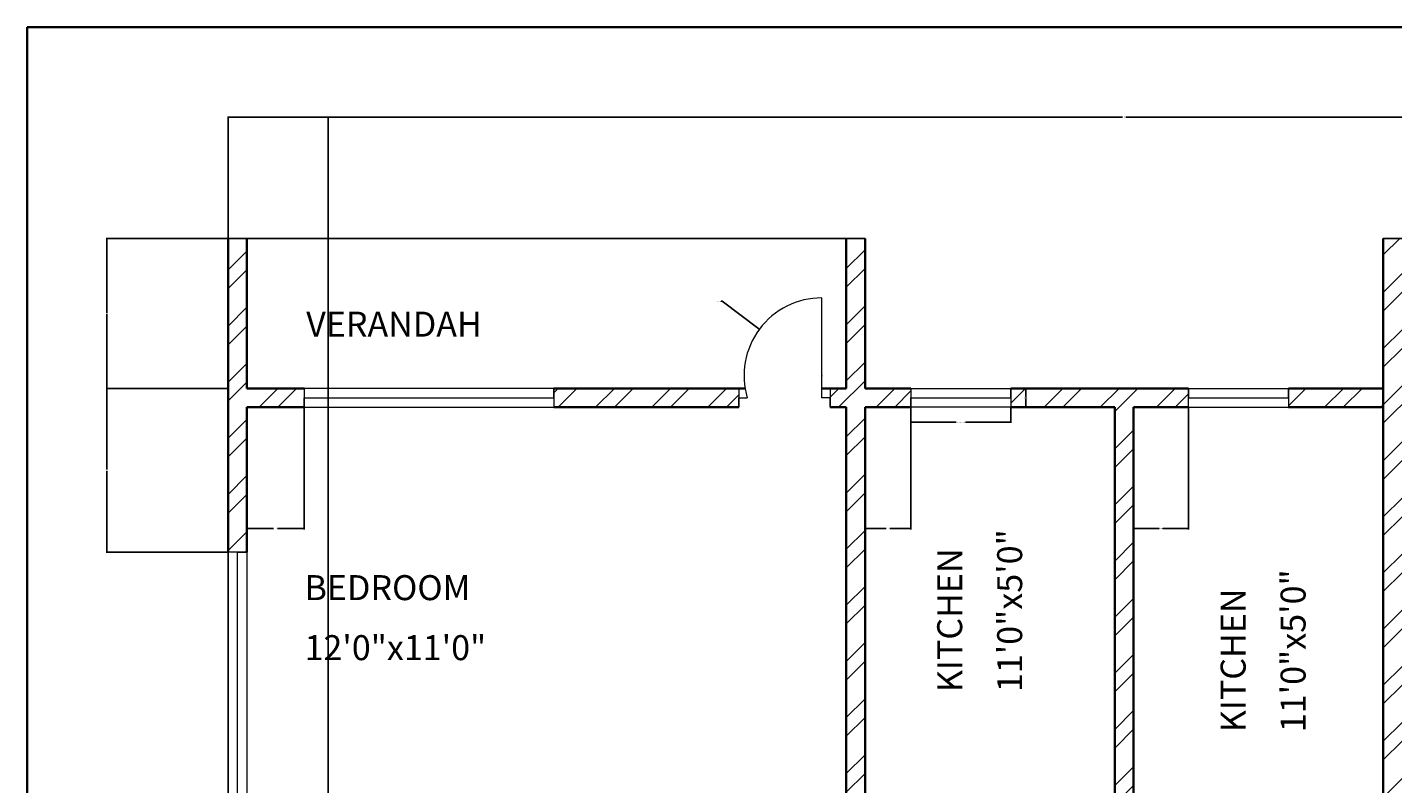
# Model space of a CAD drawing. Units: inches. Extents: x 2271 to 2815, y 1169 to 1838.
# Tile 3 of 4: x 2271 to 2599, y 1657 to 1838. Entities that reach past the tile are written whole.
import ezdxf

# ---------------------------------------------------------------- set-up
doc = ezdxf.new("R2010")
doc.units = ezdxf.units.IN
for name, color, linetype, lineweight in [('A-ANNO-DIMS', 2, 'Continuous', 18), ('A-ANNO-TTLB', 7, 'Continuous', 35), ('A-AREA-IDEN', 7, 'Continuous', 18), ('A-DOOR', 11, 'Continuous', 18), ('A-FLOR-EDGE', 7, 'Continuous', 25), ('A-GLAZ', 181, 'Continuous', 18), ('A-WALL', 7, 'Continuous', 35)]:
    doc.layers.add(name, color=color, linetype=linetype, lineweight=lineweight)
doc.layers.add('A-WALL-PATT', color=9, linetype='Continuous', lineweight=13, true_color=0xafd9aa)
doc.styles.get("Standard").update_dxf_attribs({"font": 'arial.ttf'})
doc.dimstyles.get("Standard").update_dxf_attribs({"dimtxt": 0.18, "dimasz": 0.18, "dimexe": 0.18, "dimexo": 0.0625, "dimgap": 0.09, "dimtad": 0, "dimtih": 1, "dimtoh": 1, "dimdec": 4, "dimzin": 0, "dimdsep": 46, "dimtxsty": 'Standard', "dimcen": 0.09, "dimadec": 0, "dimazin": 0, "dimtfac": 1, "dimtdec": 4, "dimtofl": 0, "dimtmove": 0, "dimatfit": 3, "dimfxl": 1, "dimtolj": 1, "dimtzin": 0, "dimarcsym": 0})

# ---------------------------------------------------------------- blocks, each defined once
blk = doc.blocks.new('WIN-60IN')
for p, q in [((0, 4.5), (0, 0)), ((60, 4.5), (0, 4.5)), ((60, 2.25), (60, 4.5)), ((60, 4.5), (60, 0)), ((0, 0), (0, 2.25)), ((0, 2.25), (60, 2.25)), ((0, 0), (60, 0))]:
    blk.add_line(p, q)
blk = doc.blocks.new('WIN-24IN')
for p, q in [((0, 4.5), (0, 0)), ((0, 4.5), (24, 4.5)), ((24, 2.25), (24, 4.5)), ((24, 4.5), (24, 0)), ((0, 0), (0, 2.25)), ((0, 2.25), (24, 2.25)), ((24, 0), (0, 0))]:
    blk.add_line(p, q)
blk = doc.blocks.new('*D5')
at = {"layer": 'A-ANNO-DIMS', "color": 0, "lineweight": -2, "transparency": 16777216}
for p, q in [((2482.83, 1746.97), (2482.83, 1743.25)), ((2506.83, 1746.97), (2506.83, 1743.25)), ((2483.01, 1743.43), (2493.71, 1743.43)), ((2506.65, 1743.43), (2495.95, 1743.43))]:
    blk.add_line(p, q, dxfattribs=at)
at = {"layer": 'A-ANNO-DIMS', "color": 0, "transparency": 16777216}
for points in [[(2483.01, 1743.46), (2483.01, 1743.4), (2482.83, 1743.43)], [(2506.65, 1743.46), (2506.65, 1743.4), (2506.83, 1743.43)]]:
    blk.add_solid(points, dxfattribs=at)
at = {"layer": 'Defpoints', "color": 0, "transparency": 16777216}
for p in [(2482.83, 1747.03), (2506.83, 1747.03), (2506.83, 1743.43)]:
    blk.add_point(p, dxfattribs=at)
at = {"layer": 'A-ANNO-DIMS', "color": 0, "transparency": 16777216, "insert": (2494.83, 1743.43), "char_height": 0.18, "attachment_point": 5}
blk.add_mtext('\\A1;WINDOW 24 TYP.', dxfattribs=at)
blk = doc.blocks.new('*D6')
at = {"layer": 'A-ANNO-DIMS', "color": 0, "lineweight": -2, "transparency": 16777216}
for p, q in [((2506.89, 1751.53), (2510.61, 1751.53)), ((2510.43, 1751.35), (2510.43, 1749.46)), ((2510.43, 1747.21), (2510.43, 1749.1)), ((2506.89, 1747.03), (2510.61, 1747.03))]:
    blk.add_line(p, q, dxfattribs=at)
at = {"layer": 'A-ANNO-DIMS', "color": 0, "transparency": 16777216}
for points in [[(2510.4, 1751.35), (2510.46, 1751.35), (2510.43, 1751.53)], [(2510.4, 1747.21), (2510.46, 1747.21), (2510.43, 1747.03)]]:
    blk.add_solid(points, dxfattribs=at)
at = {"layer": 'Defpoints', "color": 0, "transparency": 16777216}
for p in [(2506.83, 1751.53), (2510.43, 1751.53), (2506.83, 1747.03)]:
    blk.add_point(p, dxfattribs=at)
at = {"layer": 'A-ANNO-DIMS', "color": 0, "transparency": 16777216, "insert": (2510.43, 1749.28), "char_height": 0.18, "attachment_point": 5}
blk.add_mtext('\\A1;5 TYP.', dxfattribs=at)
blk = doc.blocks.new('*D7')
at = {"layer": 'A-ANNO-DIMS', "color": 0, "lineweight": -2, "transparency": 16777216}
for p, q in [((2318.8, 1787.59), (2318.8, 1816.86)), ((2318.98, 1816.68), (2533.65, 1816.68)), ((2749.12, 1816.68), (2534.45, 1816.68)), ((2749.3, 1787.59), (2749.3, 1816.86))]:
    blk.add_line(p, q, dxfattribs=at)
at = {"layer": 'A-ANNO-DIMS', "color": 0, "transparency": 16777216}
for points in [[(2318.98, 1816.71), (2318.98, 1816.65), (2318.8, 1816.68)], [(2749.12, 1816.71), (2749.12, 1816.65), (2749.3, 1816.68)]]:
    blk.add_solid(points, dxfattribs=at)
at = {"layer": 'Defpoints', "color": 0, "transparency": 16777216}
for p in [(2749.3, 1816.68), (2318.8, 1787.53), (2749.3, 1787.53)]:
    blk.add_point(p, dxfattribs=at)
at = {"layer": 'A-ANNO-DIMS', "color": 0, "transparency": 16777216, "insert": (2534.05, 1816.68), "char_height": 0.18, "attachment_point": 5}
blk.add_mtext('\\A1;430.5', dxfattribs=at)
blk = doc.blocks.new('*D21')
at = {"layer": 'A-ANNO-DIMS', "color": 0, "lineweight": -2, "transparency": 16777216}
for p, q in [((2318.74, 1751.53), (2289.47, 1751.53)), ((2289.65, 1751.35), (2289.65, 1732.06)), ((2289.65, 1712.4), (2289.65, 1731.69)), ((2318.74, 1712.22), (2289.47, 1712.22))]:
    blk.add_line(p, q, dxfattribs=at)
at = {"layer": 'A-ANNO-DIMS', "color": 0, "transparency": 16777216}
for points in [[(2289.62, 1751.35), (2289.68, 1751.35), (2289.65, 1751.53)], [(2289.62, 1712.4), (2289.68, 1712.4), (2289.65, 1712.22)]]:
    blk.add_solid(points, dxfattribs=at)
at = {"layer": 'Defpoints', "color": 0, "transparency": 16777216}
for p in [(2289.65, 1751.53), (2318.8, 1751.53), (2318.8, 1712.22)]:
    blk.add_point(p, dxfattribs=at)
at = {"layer": 'A-ANNO-DIMS', "color": 0, "transparency": 16777216, "insert": (2289.65, 1731.87), "char_height": 0.18, "attachment_point": 5}
blk.add_mtext('\\A1;39.31', dxfattribs=at)
blk = doc.blocks.new('*D22')
at = {"layer": 'A-ANNO-DIMS', "color": 0, "lineweight": -2, "transparency": 16777216}
for p, q in [((2318.74, 1787.53), (2289.47, 1787.53)), ((2289.65, 1787.35), (2289.65, 1769.71)), ((2289.65, 1751.71), (2289.65, 1769.35)), ((2318.74, 1751.53), (2289.47, 1751.53))]:
    blk.add_line(p, q, dxfattribs=at)
at = {"layer": 'A-ANNO-DIMS', "color": 0, "transparency": 16777216}
for points in [[(2289.62, 1787.35), (2289.68, 1787.35), (2289.65, 1787.53)], [(2289.62, 1751.71), (2289.68, 1751.71), (2289.65, 1751.53)]]:
    blk.add_solid(points, dxfattribs=at)
at = {"layer": 'Defpoints', "color": 0, "transparency": 16777216}
for p in [(2289.65, 1787.53), (2318.8, 1787.53), (2318.8, 1751.53)]:
    blk.add_point(p, dxfattribs=at)
at = {"layer": 'A-ANNO-DIMS', "color": 0, "transparency": 16777216, "insert": (2289.65, 1769.53), "char_height": 0.18, "attachment_point": 5}
blk.add_mtext('\\A1;36', dxfattribs=at)
blk = doc.blocks.new('*D23')
at = {"layer": 'A-ANNO-DIMS', "color": 0, "lineweight": -2, "transparency": 16777216}
for p, q in [((2318.8, 1433.59), (2318.8, 1816.86)), ((2318.98, 1816.68), (2330.58, 1816.68)), ((2342.62, 1816.68), (2331.02, 1816.68)), ((2342.8, 1433.59), (2342.8, 1816.86))]:
    blk.add_line(p, q, dxfattribs=at)
at = {"layer": 'A-ANNO-DIMS', "color": 0, "transparency": 16777216}
for points in [[(2318.98, 1816.71), (2318.98, 1816.65), (2318.8, 1816.68)], [(2342.62, 1816.71), (2342.62, 1816.65), (2342.8, 1816.68)]]:
    blk.add_solid(points, dxfattribs=at)
at = {"layer": 'Defpoints', "color": 0, "transparency": 16777216}
for p in [(2342.8, 1816.68), (2318.8, 1433.53), (2342.8, 1433.53)]:
    blk.add_point(p, dxfattribs=at)
at = {"layer": 'A-ANNO-DIMS', "color": 0, "transparency": 16777216, "insert": (2330.8, 1816.68), "char_height": 0.18, "attachment_point": 5}
blk.add_mtext('\\A1;24', dxfattribs=at)
blk = doc.blocks.new('*D26')
at = {"layer": 'A-ANNO-DIMS', "color": 0, "lineweight": -2, "transparency": 16777216}
for p, q in [((2323.3, 1746.97), (2323.3, 1717.7)), ((2337.06, 1746.97), (2337.06, 1717.7)), ((2323.48, 1717.88), (2329.72, 1717.88)), ((2336.88, 1717.88), (2330.63, 1717.88))]:
    blk.add_line(p, q, dxfattribs=at)
at = {"layer": 'A-ANNO-DIMS', "color": 0, "transparency": 16777216}
for points in [[(2323.48, 1717.91), (2323.48, 1717.85), (2323.3, 1717.88)], [(2336.88, 1717.91), (2336.88, 1717.85), (2337.06, 1717.88)]]:
    blk.add_solid(points, dxfattribs=at)
at = {"layer": 'Defpoints', "color": 0, "transparency": 16777216}
for p in [(2323.3, 1747.03), (2337.06, 1747.03), (2323.3, 1717.88)]:
    blk.add_point(p, dxfattribs=at)
at = {"layer": 'A-ANNO-DIMS', "color": 0, "transparency": 16777216, "insert": (2330.18, 1717.88), "char_height": 0.18, "attachment_point": 5}
blk.add_mtext('\\A1;13.757', dxfattribs=at)
blk = doc.blocks.new('*D27')
at = {"layer": 'A-ANNO-DIMS', "color": 0, "lineweight": -2, "transparency": 16777216}
for p, q in [((2471.8, 1746.97), (2471.8, 1717.7)), ((2482.83, 1746.97), (2482.83, 1717.7)), ((2471.98, 1717.88), (2476.86, 1717.88)), ((2482.65, 1717.88), (2477.77, 1717.88))]:
    blk.add_line(p, q, dxfattribs=at)
at = {"layer": 'A-ANNO-DIMS', "color": 0, "transparency": 16777216}
for points in [[(2471.98, 1717.91), (2471.98, 1717.85), (2471.8, 1717.88)], [(2482.65, 1717.91), (2482.65, 1717.85), (2482.83, 1717.88)]]:
    blk.add_solid(points, dxfattribs=at)
at = {"layer": 'Defpoints', "color": 0, "transparency": 16777216}
for p in [(2471.8, 1747.03), (2482.83, 1747.03), (2471.8, 1717.88)]:
    blk.add_point(p, dxfattribs=at)
at = {"layer": 'A-ANNO-DIMS', "color": 0, "transparency": 16777216, "insert": (2477.31, 1717.88), "char_height": 0.18, "attachment_point": 5}
blk.add_mtext('\\A1;11.027', dxfattribs=at)
blk = doc.blocks.new('*D28')
at = {"layer": 'A-ANNO-DIMS', "color": 0, "lineweight": -2, "transparency": 16777216}
for p, q in [((2536.3, 1746.97), (2536.3, 1717.7)), ((2549.52, 1746.97), (2549.52, 1717.7)), ((2536.48, 1717.88), (2542.45, 1717.88)), ((2549.34, 1717.88), (2543.36, 1717.88))]:
    blk.add_line(p, q, dxfattribs=at)
at = {"layer": 'A-ANNO-DIMS', "color": 0, "transparency": 16777216}
for points in [[(2536.48, 1717.91), (2536.48, 1717.85), (2536.3, 1717.88)], [(2549.34, 1717.91), (2549.34, 1717.85), (2549.52, 1717.88)]]:
    blk.add_solid(points, dxfattribs=at)
at = {"layer": 'Defpoints', "color": 0, "transparency": 16777216}
for p in [(2536.3, 1747.03), (2549.52, 1747.03), (2536.3, 1717.88)]:
    blk.add_point(p, dxfattribs=at)
at = {"layer": 'A-ANNO-DIMS', "color": 0, "transparency": 16777216, "insert": (2542.91, 1717.88), "char_height": 0.18, "attachment_point": 5}
blk.add_mtext('\\A1;13.218', dxfattribs=at)
blk = doc.blocks.new('*D46')
at = {"layer": 'A-ANNO-DIMS', "color": 0, "lineweight": -2, "transparency": 16777216}
for p, q in [((2437.27, 1772.48), (2437.45, 1772.48)), ((2437.45, 1772.48), (2446.29, 1765.88)), ((2461.32, 1754.59), (2461.5, 1754.59)), ((2461.41, 1754.5), (2461.41, 1754.68))]:
    blk.add_line(p, q, dxfattribs=at)
at = {"layer": 'A-ANNO-DIMS', "color": 0, "transparency": 16777216}
blk.add_solid([(2446.31, 1765.91), (2446.27, 1765.86), (2446.44, 1765.77)], dxfattribs=at)
at = {"layer": 'Defpoints', "color": 0, "transparency": 16777216}
for p in [(2446.44, 1765.77), (2461.41, 1754.59)]:
    blk.add_point(p, dxfattribs=at)
at = {"layer": 'A-ANNO-DIMS', "color": 0, "transparency": 16777216, "insert": (2436.79, 1772.48), "char_height": 0.18, "attachment_point": 5}
blk.add_mtext('\\A1;R18.69', dxfattribs=at)

msp = doc.modelspace()

# ---------------------------------------------------------------- hatches: boundary and pattern name
at = {"layer": 'A-WALL-PATT'}
h = msp.add_hatch(dxfattribs=at)
h.set_pattern_fill('ANSI32', color=256)
h.paths.add_polyline_path([(2441.4917, 1751.5314), (2397.0578, 1751.5314), (2397.0578, 1747.0314), (2441.4917, 1747.0314), (2441.4917, 1749.2814)])
h.paths.add_polyline_path([(2471.8006, 1787.5314), (2467.3006, 1787.5314), (2467.3006, 1783.0314), (2467.3006, 1751.5314), (2463.4131, 1751.5314), (2463.4131, 1747.0314), (2467.3006, 1747.0314), (2467.3006, 1615.0314), (2465.0606, 1615.0314), (2465.0606, 1610.5314), (2474.7192, 1610.5314), (2474.7192, 1612.7814), (2474.7192, 1615.0314), (2471.8006, 1615.0314), (2471.8006, 1747.0314), (2482.8275, 1747.0314), (2482.8275, 1749.2814), (2482.8275, 1751.5314), (2471.8006, 1751.5314)])
h.paths.add_polyline_path([(2549.5185, 1751.5314), (2506.8275, 1751.5314), (2506.8275, 1747.0314), (2531.8006, 1747.0314), (2531.8006, 1615.0314), (2496.0724, 1615.0314), (2496.0724, 1610.5314), (2531.8006, 1610.5314), (2531.8006, 1458.2548), (2528.7405, 1458.2548), (2528.7405, 1453.7548), (2539.7806, 1453.7548), (2539.7806, 1456.0048), (2539.7806, 1458.2548), (2536.3006, 1458.2548), (2536.3006, 1610.5314), (2573.267, 1610.5314), (2573.267, 1612.5736), (2573.267, 1612.7912), (2573.267, 1615.0314), (2536.3006, 1615.0314), (2536.3006, 1747.0314), (2549.5185, 1747.0314)])
h.paths.add_polyline_path([(2600.8006, 1787.5314), (2596.3006, 1787.5314), (2596.3006, 1747.0314), (2596.3006, 1615.0314), (2593.1473, 1615.0314), (2593.1473, 1610.5314), (2603.416, 1610.5314), (2603.416, 1612.7814), (2603.416, 1615.0314), (2600.8006, 1615.0314), (2600.8006, 1747.0314), (2603.7892, 1747.0314), (2603.7892, 1749.2814), (2603.7892, 1751.5314), (2600.8006, 1751.5314)])
h.paths.add_polyline_path([(2596.3006, 1751.5314), (2573.5185, 1751.5314), (2573.5185, 1747.0314), (2596.3006, 1747.0314)])
h.paths.add_polyline_path([(2648.9302, 1749.2814), (2648.9302, 1751.5314), (2624.6394, 1751.5314), (2624.6394, 1747.0314), (2648.9302, 1747.0314)])
h.paths.add_polyline_path([(2749.3006, 1751.5314), (2749.3006, 1787.5314), (2744.8006, 1787.5314), (2744.8006, 1751.5314), (2708.9302, 1751.5314), (2708.9302, 1747.0314), (2744.8006, 1747.0314), (2744.8006, 1715.8571), (2749.3006, 1715.8571)])
h.paths.add_polyline_path([(2337.0578, 1749.2814), (2337.0578, 1751.5314), (2323.3006, 1751.5314), (2323.3006, 1787.5314), (2318.8006, 1787.5314), (2318.8006, 1751.5314), (2318.8006, 1712.2179), (2323.3006, 1712.2179), (2323.3006, 1747.0314), (2337.0578, 1747.0314)])
h.paths.add_polyline_path([(2402.757, 1615.0314), (2323.3006, 1615.0314), (2323.3006, 1652.2179), (2318.8006, 1652.2179), (2318.8006, 1610.5314), (2323.3006, 1610.5314), (2342.8006, 1610.5314), (2342.8006, 1602.42), (2347.3006, 1602.42), (2347.3006, 1610.5314), (2402.757, 1610.5314)])
h.paths.add_polyline_path([(2430.8006, 1568.5314), (2430.8006, 1610.5314), (2434.8435, 1610.5314), (2434.8435, 1612.7814), (2434.8435, 1615.0314), (2422.3947, 1615.0314), (2422.3947, 1612.7814), (2422.3947, 1610.5314), (2426.3006, 1610.5314), (2426.3006, 1568.5314), (2347.3006, 1568.5314), (2347.3006, 1578.42), (2342.8006, 1578.42), (2342.8006, 1568.5314), (2318.8006, 1568.5314), (2318.8006, 1546.0693), (2322.7121, 1546.0693), (2323.3006, 1546.0693), (2323.3006, 1564.0314), (2342.8006, 1564.0314), (2347.3006, 1564.0314), (2430.8006, 1564.0314)])
h.paths.add_polyline_path([(2430.8006, 1480.0314), (2323.3006, 1480.0314), (2323.3006, 1498.0693), (2321.0506, 1498.0693), (2318.8006, 1498.0693), (2318.8006, 1475.5314), (2342.8006, 1475.5314), (2342.8006, 1466.8218), (2347.3006, 1466.8218), (2347.3006, 1475.5314), (2426.3006, 1475.5314), (2426.3006, 1458.0149), (2430.8006, 1458.0149), (2430.8006, 1475.5314)])
h.paths.add_polyline_path([(2435.9471, 1433.5314), (2430.8006, 1433.5314), (2430.8006, 1437.7896), (2426.3006, 1437.7896), (2426.3006, 1433.5314), (2347.3006, 1433.5314), (2347.3006, 1442.8218), (2342.8006, 1442.8218), (2342.8006, 1433.5314), (2318.8006, 1433.5314), (2318.8006, 1402.3145), (2323.3006, 1402.3145), (2323.3006, 1429.0314), (2342.8006, 1429.0314), (2347.3006, 1429.0314), (2435.9471, 1429.0314)])
h.paths.add_polyline_path([(2323.3006, 1342.3145), (2321.0506, 1342.3145), (2318.8006, 1342.3145), (2318.8006, 1304.5314), (2318.8006, 1268.5314), (2323.3006, 1268.5314), (2323.3006, 1304.5314), (2333.4662, 1304.5314), (2333.4662, 1306.7814), (2333.4662, 1309.0314), (2323.3006, 1309.0314)])
h.paths.add_polyline_path([(2437.8933, 1306.7814), (2437.8933, 1309.0314), (2393.4662, 1309.0314), (2393.4662, 1304.5314), (2437.8933, 1304.5314)])
h.paths.add_polyline_path([(2471.8006, 1453.7548), (2493.7895, 1453.7548), (2493.7895, 1456.0048), (2493.7895, 1458.2548), (2467.3006, 1458.2548), (2467.3006, 1433.5314), (2463.7134, 1433.5314), (2463.7134, 1431.2814), (2463.7134, 1429.0314), (2467.3006, 1429.0314), (2467.3006, 1309.0314), (2462.3197, 1309.0314), (2462.3197, 1304.5314), (2467.3006, 1304.5314), (2467.3006, 1268.5314), (2471.8006, 1268.5314), (2495.9201, 1268.5314), (2495.9201, 1270.7814), (2495.9201, 1273.0314), (2471.8006, 1273.0314), (2471.8006, 1309.0314)])
h.paths.add_polyline_path([(2600.8006, 1458.2548), (2570.4818, 1458.2548), (2570.4818, 1453.7548), (2596.3006, 1453.7548), (2596.3006, 1429.0314), (2596.3006, 1273.0314), (2555.9201, 1273.0314), (2555.9201, 1268.5314), (2596.3006, 1268.5314), (2600.8006, 1268.5314), (2600.8006, 1304.5314), (2604.5593, 1304.5314), (2604.5593, 1306.7814), (2604.5593, 1309.0314), (2600.8006, 1309.0314), (2600.8006, 1429.0314)])
h.paths.add_polyline_path([(2667.0861, 1309.0314), (2627.2, 1309.0314), (2627.2, 1304.5314), (2667.0861, 1304.5314)])
h.paths.add_polyline_path([(2749.3006, 1309.0314), (2749.3006, 1337.3095), (2744.8006, 1337.3095), (2744.8006, 1309.0314), (2727.0861, 1309.0314), (2727.0861, 1306.7814), (2727.0861, 1304.5314), (2744.8006, 1304.5314), (2744.8006, 1268.5314), (2749.3006, 1268.5314), (2749.3006, 1304.5314)])
h.paths.add_polyline_path([(2749.3006, 1433.5314), (2725.3006, 1433.5314), (2725.3006, 1442.7202), (2720.8006, 1442.7202), (2720.8006, 1433.5314), (2636.8006, 1433.5314), (2636.8006, 1437.8287), (2634.5506, 1437.8287), (2632.3006, 1437.8287), (2632.3006, 1433.5314), (2630.1129, 1433.5314), (2630.1129, 1429.0314), (2744.8006, 1429.0314), (2744.8006, 1397.3095), (2749.3006, 1397.3095)])
h.paths.add_polyline_path([(2749.3006, 1480.0314), (2749.3006, 1502.0415), (2744.8006, 1502.0415), (2744.8006, 1480.0314), (2720.8006, 1480.0314), (2632.3006, 1480.0314), (2632.3006, 1457.7851), (2636.8006, 1457.7851), (2636.8006, 1475.5314), (2720.8006, 1475.5314), (2720.8006, 1466.7202), (2725.3006, 1466.7202), (2725.3006, 1475.5314), (2749.3006, 1475.5314)])
h.paths.add_polyline_path([(2749.3006, 1568.5314), (2725.3006, 1568.5314), (2725.3006, 1578.9125), (2720.8006, 1578.9125), (2720.8006, 1568.5314), (2641.8006, 1568.5314), (2641.8006, 1610.5314), (2645.4823, 1610.5314), (2645.4823, 1612.7814), (2645.4823, 1615.0314), (2631.895, 1615.0314), (2631.895, 1610.5314), (2637.3006, 1610.5314), (2637.3006, 1568.5314), (2637.3006, 1564.0314), (2720.8006, 1564.0314), (2725.3006, 1564.0314), (2744.8006, 1564.0314), (2744.8006, 1550.0415), (2747.0506, 1550.0415), (2749.3006, 1550.0415)])
h.paths.add_polyline_path([(2749.3006, 1655.8571), (2744.8006, 1655.8571), (2744.8006, 1615.0314), (2668.3453, 1615.0314), (2668.3453, 1610.5314), (2720.8006, 1610.5314), (2720.8006, 1602.9125), (2725.3006, 1602.9125), (2725.3006, 1610.5314), (2749.3006, 1610.5314)])
h.paths.add_polyline_path([(2512.9815, 1676.2212), (2512.9815, 1716.3099), (2486.1477, 1716.3099), (2486.1477, 1676.2212)], flags=9)

# ---------------------------------------------------------------- linework, layer by layer
at = {"layer": 'A-ANNO-TTLB'}
msp.add_lwpolyline([(2270.5512, 1838.2339), (2814.8691, 1838.2339), (2814.8691, 1168.8883), (2270.5512, 1168.8883)], close=True, dxfattribs=at)
at = {"layer": 'A-DOOR'}
for p, q in [((2461.4131, 1749.2814), (2461.4131, 1773.2814)), ((2441.4917, 1751.5314), (2441.4917, 1747.0314)), ((2463.4131, 1751.5314), (2463.4131, 1747.0314)), ((2441.4917, 1747.0314), (2441.4917, 1749.2814)), ((2441.4917, 1749.2814), (2443.4917, 1749.2814)), ((2463.4131, 1749.2814), (2461.4131, 1749.2814)), ((2463.4131, 1747.0314), (2463.4131, 1749.2814))]:
    msp.add_line(p, q, dxfattribs=at)
msp.add_arc((2461.4131, 1754.5902), 18.6912, 90, 196.500677, dxfattribs=at)
at = {"layer": 'A-FLOR-EDGE'}
for p, q in [((2318.8006, 1787.5314), (2471.8006, 1787.5314)), ((2749.3006, 1787.5314), (2596.3006, 1787.5314))]:
    msp.add_line(p, q, dxfattribs=at)
at = {"layer": 'A-GLAZ'}
for p, q in [((2549.5185, 1747.0314), (2549.5185, 1751.5314)), ((2549.5185, 1751.5314), (2549.5185, 1749.2814)), ((2549.5185, 1751.5314), (2574.0026, 1751.5314)), ((2573.5185, 1749.2814), (2573.5185, 1751.5314)), ((2573.5185, 1751.5314), (2573.5185, 1747.0314)), ((2549.5185, 1749.2814), (2573.5185, 1749.2814)), ((2549.5185, 1747.0314), (2573.5185, 1747.0314))]:
    msp.add_line(p, q, dxfattribs=at)
at = {"layer": 'A-WALL'}
for p, q in [((2318.8006, 1751.5314), (2318.8006, 1787.5314)), ((2323.3006, 1787.5314), (2323.3006, 1751.5314)), ((2467.3006, 1751.5314), (2467.3006, 1787.5314)), ((2467.3006, 1787.5314), (2467.3006, 1783.0314)), ((2471.8006, 1787.5314), (2471.8006, 1751.5314)), ((2596.3006, 1787.5314), (2596.3006, 1747.0314)), ((2318.8006, 1751.5314), (2318.8006, 1712.2179)), ((2323.3006, 1751.5314), (2337.0578, 1751.5314)), ((2397.0578, 1751.5314), (2442.9739, 1751.5314)), ((2461.4131, 1751.5314), (2467.3006, 1751.5314)), ((2471.8006, 1751.5314), (2482.8275, 1751.5314)), ((2506.8275, 1751.5314), (2549.5185, 1751.5314)), ((2573.5185, 1751.5314), (2596.3006, 1751.5314)), ((2323.3006, 1747.0314), (2337.0578, 1747.0314)), ((2323.3006, 1747.0314), (2323.3006, 1712.2179)), ((2397.0578, 1747.0314), (2441.4917, 1747.0314)), ((2463.4131, 1747.0314), (2467.3006, 1747.0314)), ((2467.3006, 1747.0314), (2467.3006, 1615.0314)), ((2471.8006, 1747.0314), (2471.8006, 1615.0314)), ((2471.8006, 1747.0314), (2482.8275, 1747.0314)), ((2506.8275, 1747.0314), (2531.8006, 1747.0314)), ((2531.8006, 1747.0314), (2531.8006, 1615.0314)), ((2536.3006, 1747.0314), (2536.3006, 1615.0314)), ((2536.3006, 1747.0314), (2549.5185, 1747.0314)), ((2573.5185, 1747.0314), (2596.3006, 1747.0314)), ((2596.3006, 1747.0314), (2596.3006, 1615.0314))]:
    msp.add_line(p, q, dxfattribs=at)

# ---------------------------------------------------------------- block references
at = {"layer": 'A-GLAZ'}
for name, p in [('WIN-60IN', (2337.058, 1747.031)), ('WIN-24IN', (2482.827, 1747.031))]:
    msp.add_blockref(name, p, dxfattribs=at)
at = {"layer": 'A-GLAZ', "extrusion": (0, 0, -1), "zscale": -1, "rotation": 90}
msp.add_blockref('WIN-60IN', (-2318.8001, 1652.2181), dxfattribs=at)

# ---------------------------------------------------------------- texts
at = {"layer": 'A-AREA-IDEN', "char_height": 6, "attachment_point": 1, "line_spacing_factor": 1.44}
for s, width, insert in [('VERANDAH', 202.405664, (2337.5496, 1769.9702)), ('BEDROOM\\P12\'0"x11\'0"', 161.979408, (2337.1478, 1706.7139))]:
    msp.add_mtext_dynamic_manual_height_columns(s, width=width, gutter_width=12.5, heights=[0], dxfattribs=dict(at, insert=insert))
at = {"layer": 'A-AREA-IDEN', "char_height": 6, "attachment_point": 1, "rotation": 90, "line_spacing_factor": 1.44}
for width, insert in [(227.63428, (2489.1333, 1678.6339)), (157.942047, (2557.2185, 1669.0129))]:
    msp.add_mtext_dynamic_manual_height_columns('KITCHEN\\P11\'0"x5\'0"', width=width, gutter_width=12.5, heights=[0], dxfattribs=dict(at, insert=insert))

# ---------------------------------------------------------------- dimensions: what is measured, and where the dimension line sits
at = {"layer": 'A-ANNO-DIMS'}
for base, p1, p2, override, picture, middle in [((2749.3006, 1816.6814), (2318.8006, 1787.5314), (2749.3006, 1787.5314), {"dimdec": 1, "dimlfac": 1, "dimrnd": 0, "dimzin": 0, "dimdsep": 46, "dimlunit": 2}, '*D7', (2534.0506, 1816.6814)), ((2342.8006, 1816.6814), (2318.8006, 1433.5314), (2342.8006, 1433.5314), {"dimdec": 0, "dimlfac": 1, "dimrnd": 0, "dimzin": 0, "dimdsep": 46, "dimlunit": 2}, '*D23', (2330.8006, 1816.6814))]:
    dim = msp.add_linear_dim(base=base, p1=p1, p2=p2, dimstyle='Standard', override=override, dxfattribs=at)
    dim.commit()
    dim.dimension.update_dxf_attribs({"geometry": picture, "text_midpoint": middle})
for base, p1, p2, angle, override, picture, middle in [((2289.6506, 1787.5314), (2318.8006, 1751.5314), (2318.8006, 1787.5314), 90, {"dimdec": 0, "dimlfac": 1, "dimrnd": 0, "dimzin": 0, "dimdsep": 46, "dimlunit": 2}, '*D22', (2289.6506, 1769.5314)), ((2289.6506, 1751.5314), (2318.8006, 1712.2179), (2318.8006, 1751.5314), 90, {"dimdec": 2, "dimlfac": 1, "dimrnd": 0, "dimzin": 0, "dimdsep": 46, "dimlunit": 2}, '*D21', (2289.6506, 1731.8747)), ((2323.3006, 1717.8814), (2337.0578, 1747.0314), (2323.3006, 1747.0314), 180, {"dimdec": 3, "dimlfac": 1, "dimrnd": 0, "dimzin": 0, "dimdsep": 46, "dimlunit": 2}, '*D26', (2330.1792, 1717.8814)), ((2471.8006, 1717.8814), (2482.8275, 1747.0314), (2471.8006, 1747.0314), 180, {"dimdec": 3, "dimlfac": 1, "dimrnd": 0, "dimzin": 0, "dimdsep": 46, "dimlunit": 2}, '*D27', (2477.314, 1717.8814)), ((2536.3006, 1717.8814), (2549.5185, 1747.0314), (2536.3006, 1747.0314), 180, {"dimdec": 3, "dimlfac": 1, "dimrnd": 0, "dimzin": 0, "dimdsep": 46, "dimlunit": 2}, '*D28', (2542.9095, 1717.8814))]:
    dim = msp.add_linear_dim(base=base, p1=p1, p2=p2, angle=angle, dimstyle='Standard', override=override, dxfattribs=at)
    dim.commit()
    dim.dimension.update_dxf_attribs({"geometry": picture, "text_midpoint": middle})
dim = msp.add_radius_dim(center=(2461.4131, 1754.5902), mpoint=(2446.437, 1765.774), dimstyle='Standard', override={"dimdec": 2, "dimlfac": 1, "dimrnd": 0, "dimzin": 0, "dimdsep": 46, "dimlunit": 2}, dxfattribs=at)
dim.commit()
dim.dimension.update_dxf_attribs({"geometry": '*D46', "text_midpoint": (2436.7913, 1772.4843), "dimtype": 164})
dim = msp.add_linear_dim(base=(2510.4274603539, 1751.5314174086), p1=(2506.8274603539, 1747.0314174086), p2=(2506.8274603539, 1751.5314174086), angle=90, text='<> TYP.', dimstyle='Standard', override={"dimdec": 0, "dimlfac": 1, "dimrnd": 0, "dimzin": 0, "dimdsep": 46, "dimlunit": 2}, dxfattribs=at)
dim.commit()
dim.dimension.update_dxf_attribs({"geometry": '*D6', "text_midpoint": (2510.4274603539, 1749.2814174086)})
dim = msp.add_linear_dim(base=(2506.8275, 1743.4314), p1=(2482.8275, 1747.0314), p2=(2506.8275, 1747.0314), text='WINDOW <> TYP.', dimstyle='Standard', override={"dimdec": 0, "dimlfac": 1, "dimrnd": 0, "dimzin": 0, "dimdsep": 46, "dimlunit": 2}, dxfattribs=at)
dim.commit()
dim.dimension.update_dxf_attribs({"geometry": '*D5', "text_midpoint": (2494.8275, 1743.4314)})

doc.saveas('drawing.dxf')
